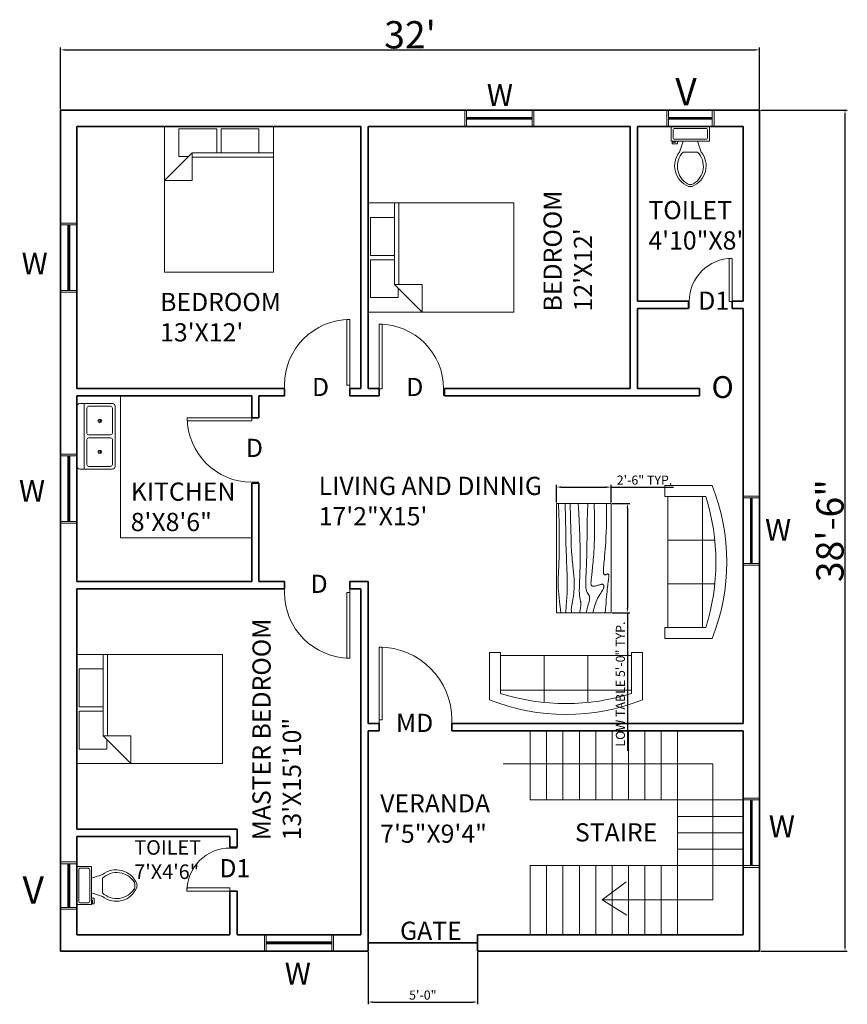
# Model space of a CAD drawing. Units: inches. Extents: x 1662 to 23131, y 1265 to 19127.
# Tile 4 of 26: x 8519 to 8974, y 5033 to 5574. Entities that reach past the tile are written whole.
import ezdxf

# ---------------------------------------------------------------- set-up
doc = ezdxf.new("R2010")
doc.units = ezdxf.units.IN
for name, color, linetype, lineweight in [('A-ANNO-DIMS', 4, 'Continuous', 18), ('A-ANNO-IDEN', 7, 'Continuous', 18), ('A-AREA-IDEN', 7, 'Continuous', 18), ('A-DOOR', 3, 'Continuous', 18), ('A-FLOR-CASE', 8, 'Continuous', 18), ('A-FLOR-FIXT', 9, 'Continuous', 18), ('A-FLOR-STRS', 7, 'Continuous', 18), ('A-FURN', 8, 'Continuous', 18), ('A-GLAZ', 4, 'Continuous', 18), ('A-WALL', 7, 'Continuous', 35)]:
    doc.layers.add(name, color=color, linetype=linetype, lineweight=lineweight)
doc.styles.get("Standard").update_dxf_attribs({"font": 'arial.ttf'})
doc.dimstyles.new('ISO-25', dxfattribs={"dimtxt": 5, "dimasz": 2.5, "dimexe": 1.25, "dimexo": 0.625, "dimtad": 1, "dimlunit": 3, "dimtxsty": 'Standard', "dimcen": 2.5, "dimadec": 0, "dimazin": 0, "dimtfac": 1, "dimtmove": 0, "dimatfit": 3, "dimfxl": 1, "dimarcsym": 0})

# ---------------------------------------------------------------- blocks, each defined once
blk = doc.blocks.new('Table - Rectangular Woodgrain 60 x 30 in.')
for p, q in [((0, 0), (0, -30)), ((60, 0), (0, 0)), ((60, -30), (60, 0)), ((0, -30), (60, -30))]:
    blk.add_line(p, q)
for points in [[(0, -2.4), (4.8155, -2.418), (9.0302, -2.4688), (12.709, -2.5477), (15.9167, -2.65), (18.7181, -2.7711), (21.1781, -2.9063), (23.3616, -3.0508), (25.3333, -3.2), (27.1477, -3.3495), (28.8172, -3.4958), (30.3437, -3.636), (31.7291, -3.7667), (32.9756, -3.8849), (34.0849, -3.9875), (35.059, -4.0714), (35.9, -4.1334), (36.6114, -4.1711), (37.2041, -4.1854), (37.6906, -4.1779), (38.0833, -4.15), (38.3948, -4.1034), (38.6375, -4.0396), (38.8239, -3.9602), (38.9666, -3.8667), (39.0764, -3.7608), (39.1573, -3.6448), (39.2116, -3.521), (39.2416, -3.3917), (39.2498, -3.2593), (39.2385, -3.1261), (39.21, -2.9944), (39.1666, -2.8667), (39.111, -2.7447), (39.0468, -2.6281), (38.978, -2.5163), (38.9083, -2.4083), (38.8418, -2.3035), (38.7823, -2.201), (38.7337, -2.1001), (38.7, -2), (38.6844, -1.9003), (38.6875, -1.8021), (38.7094, -1.707), (38.75, -1.6167), (38.8094, -1.5326), (38.8875, -1.4563), (38.9844, -1.3893), (39.1, -1.3333), (39.2351, -1.2896), (39.3937, -1.2583), (39.5804, -1.2396), (39.8, -1.2333), (40.057, -1.2396), (40.3562, -1.2583), (40.7023, -1.2896), (41.1, -1.3333), (41.5547, -1.3895), (42.0755, -1.4573), (42.6721, -1.5361), (43.3542, -1.625), (44.1316, -1.7233), (45.014, -1.8302), (46.0114, -1.9449), (47.1333, -2.0667), (48.3862, -2.1947), (49.7625, -2.3281), (51.2513, -2.4663), (52.8416, -2.6083), (54.5226, -2.7535), (56.2833, -2.9011), (58.1127, -3.0501), (60, -3.2)], [(0, -9.2), (6.5759, -9.0858), (11.9385, -9.0365), (16.2527, -9.0418), (19.6833, -9.0917), (22.3952, -9.1759), (24.5531, -9.2844), (26.322, -9.4069), (27.8666, -9.5333), (29.3241, -9.6553), (30.7203, -9.7719), (32.0532, -9.8837), (33.3208, -9.9917), (34.5213, -10.0965), (35.6526, -10.199), (36.7128, -10.2999), (37.7, -10.4), (38.6129, -10.4996), (39.4531, -10.5969), (40.223, -10.6895), (40.925, -10.775), (41.5613, -10.8512), (42.1344, -10.9156), (42.6465, -10.966), (43.1, -11), (43.4976, -11.0158), (43.8437, -11.0136), (44.143, -10.9942), (44.4, -10.9583), (44.6195, -10.9069), (44.8062, -10.8406), (44.9648, -10.7603), (45.1, -10.6667), (45.2155, -10.5598), (45.3114, -10.4365), (45.3871, -10.2929), (45.4416, -10.125), (45.4743, -9.929), (45.4844, -9.7011), (45.4709, -9.4371), (45.4333, -9.1333), (45.3716, -8.7883), (45.2896, -8.4104), (45.1919, -8.0107), (45.0833, -7.6), (44.9685, -7.1893), (44.8521, -6.7896), (44.7388, -6.4117), (44.6333, -6.0667), (44.54, -5.7628), (44.4614, -5.4979), (44.4001, -5.2675), (44.3583, -5.0667), (44.3384, -4.8909), (44.3427, -4.7354), (44.3736, -4.5956), (44.4333, -4.4667), (44.5236, -4.3453), (44.6427, -4.2333), (44.7884, -4.1339), (44.9583, -4.05), (45.1501, -3.9849), (45.3614, -3.9417), (45.59, -3.9234), (45.8333, -3.9333), (46.0915, -3.9749), (46.3734, -4.0531), (46.6906, -4.1736), (47.0542, -4.3417), (47.4756, -4.5629), (47.9661, -4.8427), (48.5372, -5.1866), (49.2, -5.6), (49.9676, -6.0844), (50.8594, -6.625), (51.8965, -7.2031), (53.1, -7.8), (54.491, -8.3969), (56.0906, -8.975), (57.9199, -9.5156), (60, -10)], [(0, -12.8), (5.1847, -12.9322), (9.6213, -13.0323), (13.3963, -13.1059), (16.5958, -13.1583), (19.3063, -13.1952), (21.614, -13.2219), (23.6054, -13.2439), (25.3666, -13.2667), (26.9728, -13.2947), (28.4531, -13.3281), (29.8256, -13.3663), (31.1083, -13.4083), (32.3191, -13.4535), (33.476, -13.501), (34.597, -13.5501), (35.7, -13.6), (36.7984, -13.6497), (37.8875, -13.6979), (38.9578, -13.743), (40, -13.7833), (41.0047, -13.8174), (41.9625, -13.8438), (42.864, -13.8607), (43.7, -13.8667), (44.4631, -13.8604), (45.1552, -13.8417), (45.7801, -13.8104), (46.3416, -13.7667), (46.8439, -13.7104), (47.2906, -13.6417), (47.6858, -13.5604), (48.0333, -13.4667), (48.3375, -13.3608), (48.6042, -13.2448), (48.8396, -13.121), (49.05, -12.9917), (49.2417, -12.8593), (49.4208, -12.7261), (49.5937, -12.5944), (49.7667, -12.4667), (49.9452, -12.3451), (50.1323, -12.2313), (50.3303, -12.1268), (50.5416, -12.0333), (50.7686, -11.9524), (51.0135, -11.8854), (51.2788, -11.8341), (51.5666, -11.8), (51.8785, -11.7843), (52.2116, -11.7865), (52.562, -11.8059), (52.926, -11.8417), (53.2998, -11.8931), (53.6795, -11.9594), (54.0614, -12.0397), (54.4416, -12.1333), (54.8223, -12.2401), (55.2293, -12.3625), (55.6942, -12.5037), (56.2489, -12.6667), (56.9251, -12.8547), (57.7545, -13.0708), (58.7689, -13.3182), (60, -13.6)], [(0, -18), (5.124, -17.7273), (9.6609, -17.5057), (13.6705, -17.3303), (17.2125, -17.1958), (20.3467, -17.0973), (23.1328, -17.0297), (25.6307, -16.9878), (27.9, -16.9667), (29.9928, -16.9617), (31.9302, -16.9703), (33.7254, -16.9907), (35.3917, -17.0208), (36.9423, -17.0588), (38.3906, -17.1026), (39.7499, -17.1503), (41.0333, -17.2), (42.2519, -17.2496), (43.4073, -17.2969), (44.4986, -17.3395), (45.525, -17.375), (46.4858, -17.4012), (47.3802, -17.4156), (48.2074, -17.416), (48.9667, -17.4), (49.6583, -17.3662), (50.2872, -17.3167), (50.8595, -17.2547), (51.3812, -17.1833), (51.8584, -17.1057), (52.2971, -17.025), (52.7034, -16.9443), (53.0833, -16.8667), (53.443, -16.7951), (53.789, -16.7313), (54.128, -16.6768), (54.4666, -16.6334), (54.8115, -16.6024), (55.1693, -16.5854), (55.5465, -16.5841), (55.95, -16.6), (56.3828, -16.6337), (56.8346, -16.6823), (57.2915, -16.7418), (57.7396, -16.8084), (58.165, -16.878), (58.5539, -16.9469), (58.8924, -17.0111), (59.1666, -17.0667), (59.3679, -17.1107), (59.5078, -17.1438), (59.6032, -17.1675), (59.6708, -17.1833), (59.7275, -17.193), (59.7901, -17.1979), (59.8753, -17.1998), (60, -17.2)], [(0, -22.4), (8.0098, -22.2501), (14.4094, -22.1011), (19.4168, -21.9535), (23.25, -21.8083), (26.1269, -21.6663), (28.2656, -21.5281), (29.884, -21.3947), (31.2, -21.2667), (32.3967, -21.1448), (33.5172, -21.0292), (34.5697, -20.9198), (35.5625, -20.8167), (36.5037, -20.7198), (37.4015, -20.6292), (38.2642, -20.5448), (39.1, -20.4667), (39.9164, -20.3951), (40.7187, -20.3313), (41.5117, -20.2768), (42.3, -20.2333), (43.0883, -20.2024), (43.8812, -20.1854), (44.6836, -20.1841), (45.5, -20.2), (46.3328, -20.234), (47.1747, -20.2844), (48.0163, -20.3488), (48.8479, -20.425), (49.66, -20.5106), (50.4429, -20.6031), (51.1872, -20.7004), (51.8833, -20.8), (52.5246, -20.8999), (53.1166, -20.9995), (53.6681, -21.0983), (54.1875, -21.1958), (54.6834, -21.2919), (55.1646, -21.3859), (55.6394, -21.4777), (56.1167, -21.5667), (56.6028, -21.6515), (57.0961, -21.7266), (57.5929, -21.7852), (58.0896, -21.8208), (58.5823, -21.8268), (59.0674, -21.7964), (59.5412, -21.723), (60, -21.6)], [(0, -25.2), (8.6355, -25.0504), (15.7026, -24.9031), (21.4049, -24.7606), (25.9458, -24.625), (29.529, -24.4988), (32.3578, -24.3844), (34.6359, -24.284), (36.5667, -24.2), (38.3213, -24.1341), (39.9417, -24.0854), (41.437, -24.0523), (42.8167, -24.0333), (44.0901, -24.0268), (45.2667, -24.0313), (46.3557, -24.0451), (47.3667, -24.0667), (48.309, -24.0947), (49.1928, -24.1287), (50.0284, -24.168), (50.826, -24.2125), (51.5959, -24.2617), (52.3483, -24.3151), (53.0935, -24.3725), (53.8417, -24.4334), (54.6009, -24.497), (55.3699, -24.561), (56.1454, -24.6226), (56.9239, -24.6792), (57.7021, -24.7279), (58.4764, -24.7662), (59.2435, -24.7911), (60, -24.8)], [(0, -28.8), (5.6867, -28.6681), (10.45, -28.5698), (14.407, -28.5012), (17.675, -28.4584), (20.3711, -28.4374), (22.6125, -28.4344), (24.5164, -28.4455), (26.2, -28.4667), (27.762, -28.4947), (29.2276, -28.5281), (30.6033, -28.5663), (31.8958, -28.6084), (33.1118, -28.6535), (34.2578, -28.7011), (35.3405, -28.7501), (36.3666, -28.8), (37.3443, -28.8497), (38.288, -28.8974), (39.2137, -28.9412), (40.1375, -28.9792), (41.0753, -29.0093), (42.0432, -29.0297), (43.0572, -29.0384), (44.1333, -29.0333), (45.2936, -29.0114), (46.5843, -28.9641), (48.0579, -28.8816), (49.7666, -28.7542), (51.7629, -28.5721), (54.0989, -28.3255), (56.8272, -28.0048), (60, -27.6)]]:
    blk.add_lwpolyline(points)
blk = doc.blocks.new('Bed - Queen')
for p, q in [((0, -80.00003), (0, 0)), ((0, 0), (59.99999, 0)), ((59.99999, 0), (59.99999, -80.00003)), ((7.99999, -1.2), (28.79998, -1.2)), ((7.99999, -14.4), (7.99999, -1.2)), ((28.79998, -1.2), (28.79998, -14.4)), ((31.19999, -1.2), (51.99999, -1.2)), ((31.19999, -14.4), (31.19999, -1.2)), ((51.99999, -1.2), (51.99999, -16.4)), ((0, -14.4), (44.8, -14.4)), ((59.99999, -29.6), (44.8, -14.4)), ((44.8, -14.4), (44.8, -29.6)), ((44.8, -16.8), (0, -16.8)), ((51.99999, -16.4), (46.79936, -16.4)), ((44.8, -29.6), (59.99999, -29.6)), ((59.99999, -80.00003), (0, -80.00003))]:
    blk.add_line(p, q)
blk = doc.blocks.new('*U33')
for p, q in [((0, 0), (0, -6)), ((40, 0), (40, -6))]:
    blk.add_line(p, q)
blk.add_lwpolyline([(0, 0), (0, 40), (1.75, 40), (1.75, 0)], close=True)
blk.add_arc((0, 0), 40, 0, 90)
blk = doc.blocks.new('*U34')
for p, q in [((0, 0), (0, -6)), ((-36, 0), (-36, -6))]:
    blk.add_line(p, q)
blk.add_lwpolyline([(0, 0), (0, 36), (-1.75, 36), (-1.75, 0)], close=True)
blk.add_arc((0, 0), 36, 90, 180)
blk = doc.blocks.new('*U40')
for p, q in [((-36, 0), (-36, 6)), ((0, 0), (0, 6))]:
    blk.add_line(p, q)
blk.add_lwpolyline([(0, 0), (0, -36), (-1.75, -36), (-1.75, 0)], close=True)
blk.add_arc((0, 0), 36, 180, 270)
blk = doc.blocks.new('*U42')
for p, q in [((0, 0), (0, -100)), ((900, 0), (900, -100))]:
    blk.add_line(p, q)
blk.add_lwpolyline([(0, 0), (0, 900), (43.75, 900), (43.75, 0)], close=True)
blk.add_arc((0, 0), 900, 0, 90)
blk = doc.blocks.new('*U41')
for p, q in [((0, 0), (0, -100)), ((-900, 0), (-900, -100))]:
    blk.add_line(p, q)
blk.add_lwpolyline([(0, 0), (0, 900), (-43.75, 900), (-43.75, 0)], close=True)
blk.add_arc((0, 0), 900, 90, 180)
blk = doc.blocks.new('*U35')
for p, q in [((0, 0), (0, -100)), ((600, 0), (600, -100))]:
    blk.add_line(p, q)
blk.add_lwpolyline([(0, 0), (0, 600), (43.75, 600), (43.75, 0)], close=True)
blk.add_arc((0, 0), 600, 0, 90)
blk = doc.blocks.new('*U43')
for p, q in [((-600, 0), (-600, -100)), ((0, 0), (0, -100))]:
    blk.add_line(p, q)
blk.add_lwpolyline([(0, 0), (0, 600), (-43.75, 600), (-43.75, 0)], close=True)
blk.add_arc((0, 0), 600, 90, 180)
blk = doc.blocks.new('Sofa - Roundback 7 ft.')
for p, q in [((-12.00002, -32.4421), (-12.00003, -6.5971)), ((11.99997, -32.4421), (11.99998, -6.5971)), ((-36.000027, -34), (-36.000027, -11.4696)), ((-35.999844, -13.3819), (35.9998, -13.3819)), ((35.99998, -34), (35.99998, -11.4696)), ((-36.000027, -32.4421), (35.99998, -32.4421))]:
    blk.add_line(p, q)
for points in [[(-36.000027, -34), (-42.000027, -34), (-42.000027, -8)], [(41.99998, -8), (41.99998, -34), (35.99998, -34)]]:
    blk.add_lwpolyline(points)
for centre, radius, start, end in [((0, -114.25), 114.25, 68.43141, 111.5686), ((-0.00001, -127.1968), 121.1968, 72.72033, 107.2797)]:
    blk.add_arc(centre, radius, start, end)
blk = doc.blocks.new('Toilet - top')
for p, q in [((9.5, -6), (9.5, -2)), ((-10, -8.5), (-8, -8.5)), ((-10, -9.5), (-10, -8.5)), ((-7, -9.5), (-10, -9.5)), ((-8, -8.5), (-8, -8)), ((-7, -8), (-7, -9.5)), ((-4, -8), (-6, -14)), ((4, -8), (6, -14)), ((4, -14), (-4, -14))]:
    blk.add_line(p, q)
blk.add_lwpolyline([(10.5, -8), (10.5, 0), (-10.5, 0), (-10.5, -8)], close=True)
for points in [[(-9.5, -2), (-9.5, -6)], [(8.5, -1), (-8.5, -1)], [(-8.5, -7), (8.5, -7)]]:
    blk.add_lwpolyline(points)
for centre, radius, start, end in [((-8.62, -1.88), 0.884, 81.8699, 188.1301), ((8.62, -1.88), 0.884, 351.8699, 98.1301), ((-8.62, -6.12), 0.884, 171.8699, 278.1301), ((8.62, -6.12), 0.884, 261.8699, 8.1301), ((3.52, -21.58), 12.17, 141.4691, 247.9714), ((4.2, -21.82), 11.33, 136.3677, 238.9468), ((-3.52, -21.58), 12.17, 292.0284, 38.5307), ((-4.2, -21.82), 11.33, 301.053, 43.6321), ((0, -27.88), 4, 245.7318, 294.2682), ((0, -29), 4, 254.8605, 285.1395)]:
    blk.add_arc(centre, radius, start, end)
blk = doc.blocks.new('Sink-double - 36 in top')
for p, q in [((-18, -4), (18, -4)), ((-0.75, -18.5), (-0.75, -6.5)), ((0.75, -6.5), (0.75, -18.5))]:
    blk.add_line(p, q)
for points in [[(-16.5, 0), (16.5, 0)], [(-18, -19.5), (-18, -1.5)], [(18, -1.5), (18, -19.5)], [(-16.5, -18.5), (-16.5, -6.5)], [(-15.5, -5.5), (-1.75, -5.5)], [(1.75, -5.5), (15.5, -5.5)], [(16.5, -6.5), (16.5, -18.5)], [(16.5, -21), (-16.5, -21)], [(-1.75, -19.5), (-15.5, -19.5)], [(15.5, -19.5), (1.75, -19.5)]]:
    blk.add_lwpolyline(points)
for centre, radius in [((-8.5, -12.5), 1), ((-8.5, -12.5), 0.5), ((8.5, -12.5), 1), ((8.5, -12.5), 0.5)]:
    blk.add_circle(centre, radius)
for centre, radius, start, end in [((-16.5, -1.5), 1.5, 90, 180), ((16.5, -1.5), 1.5, 0, 90), ((-15.5, -6.5), 1, 90, 180), ((-1.75, -6.5), 1, 0, 90), ((1.75, -6.5), 1, 90, 180), ((15.5, -6.5), 1, 0, 90), ((-16.5, -19.5), 1.5, 180, 270), ((-15.5, -18.5), 1, 180, 270), ((-1.75, -18.5), 1, 270, 0), ((1.75, -18.5), 1, 180, 270), ((15.5, -18.5), 1, 270, 0), ((16.5, -19.5), 1.5, 270, 0)]:
    blk.add_arc(centre, radius, start, end)
blk = doc.blocks.new('*D44')
at = {"layer": 'A-ANNO-DIMS', "color": 0, "lineweight": -2, "transparency": 16777216}
for p, q in [((8541.92, 5525.22), (8541.92, 5558.98)), ((8544.42, 5557.73), (8923.42, 5557.73)), ((8925.92, 5525.22), (8925.92, 5558.98))]:
    blk.add_line(p, q, dxfattribs=at)
at = {"layer": 'A-ANNO-DIMS', "color": 0, "transparency": 16777216}
for points in [[(8544.42, 5558.15), (8544.42, 5557.32), (8541.92, 5557.73)], [(8923.42, 5558.15), (8923.42, 5557.32), (8925.92, 5557.73)]]:
    blk.add_solid(points, dxfattribs=at)
at = {"layer": 'Defpoints', "color": 0, "transparency": 16777216}
for p in [(8925.92, 5557.73), (8541.92, 5524.6), (8925.92, 5524.6)]:
    blk.add_point(p, dxfattribs=at)
at = {"layer": 'A-ANNO-DIMS', "color": 0, "transparency": 16777216, "insert": (8733.92, 5566.02), "char_height": 5, "attachment_point": 5}
blk.add_mtext("{\\H3x;32'}", dxfattribs=at)
blk = doc.blocks.new('*D45')
at = {"layer": 'A-ANNO-DIMS', "color": 0, "lineweight": -2, "transparency": 16777216}
for p, q in [((8926.55, 5524.6), (8974.14, 5524.6)), ((8972.89, 5065.1), (8972.89, 5522.1)), ((8926.55, 5062.6), (8974.14, 5062.6))]:
    blk.add_line(p, q, dxfattribs=at)
at = {"layer": 'A-ANNO-DIMS', "color": 0, "transparency": 16777216}
for points in [[(8972.48, 5522.1), (8973.31, 5522.1), (8972.89, 5524.6)], [(8972.48, 5065.1), (8973.31, 5065.1), (8972.89, 5062.6)]]:
    blk.add_solid(points, dxfattribs=at)
at = {"layer": 'Defpoints', "color": 0, "transparency": 16777216}
for p in [(8925.92, 5524.6), (8972.89, 5524.6), (8925.92, 5062.6)]:
    blk.add_point(p, dxfattribs=at)
at = {"layer": 'A-ANNO-DIMS', "color": 0, "transparency": 16777216, "insert": (8964.61, 5293.6), "char_height": 5, "attachment_point": 5, "rotation": 90}
blk.add_mtext('{\\H3x;38\'-6"}', dxfattribs=at)
blk = doc.blocks.new('WIN-36-J9X1')
for p, q in [((0, 9), (0, 0)), ((1, 9), (1, 0)), ((37, 9), (37, 0)), ((38, 9), (38, 0)), ((1, 5), (37, 5)), ((1, 4.5), (37, 4.5)), ((1, 4), (37, 4))]:
    blk.add_line(p, q)
blk = doc.blocks.new('VENT-24-J9X1')
for p, q in [((0, 9), (0, 0)), ((1, 9), (1, 0)), ((25, 9), (25, 0)), ((26, 9), (26, 0)), ((1, 5), (25, 5)), ((1, 4.5), (25, 4.5)), ((1, 4), (25, 4))]:
    blk.add_line(p, q)
blk = doc.blocks.new('*D169')
at = {"layer": 'A-ANNO-DIMS', "color": 0, "lineweight": -2, "transparency": 16777216}
for p, q in [((8844.96, 5308.51), (8854.58, 5308.51)), ((8853.33, 5306.01), (8853.33, 5251.01)), ((8844.96, 5248.51), (8854.58, 5248.51)), ((8853.33, 5248.51), (8853.33, 5172.58))]:
    blk.add_line(p, q, dxfattribs=at)
at = {"layer": 'A-ANNO-DIMS', "color": 0, "transparency": 16777216}
for points in [[(8852.91, 5306.01), (8853.75, 5306.01), (8853.33, 5308.51)], [(8852.91, 5251.01), (8853.75, 5251.01), (8853.33, 5248.51)]]:
    blk.add_solid(points, dxfattribs=at)
at = {"layer": 'Defpoints', "color": 0, "transparency": 16777216}
for p in [(8844.33, 5308.51), (8844.33, 5248.51), (8853.33, 5248.51)]:
    blk.add_point(p, dxfattribs=at)
at = {"layer": 'A-ANNO-DIMS', "color": 0, "transparency": 16777216, "insert": (8850.12, 5209.29), "char_height": 5, "attachment_point": 5, "rotation": 90}
blk.add_mtext('LOW TABLE 5\'-0" TYP.', dxfattribs=at)
blk = doc.blocks.new('*D170')
at = {"layer": 'A-ANNO-DIMS', "color": 0, "lineweight": -2, "transparency": 16777216}
for p, q in [((8814.33, 5309.13), (8814.33, 5318.76)), ((8844.33, 5309.13), (8844.33, 5318.76)), ((8816.83, 5317.51), (8841.83, 5317.51)), ((8844.33, 5317.51), (8878.64, 5317.51))]:
    blk.add_line(p, q, dxfattribs=at)
at = {"layer": 'A-ANNO-DIMS', "color": 0, "transparency": 16777216}
for points in [[(8816.83, 5317.92), (8816.83, 5317.09), (8814.33, 5317.51)], [(8841.83, 5317.92), (8841.83, 5317.09), (8844.33, 5317.51)]]:
    blk.add_solid(points, dxfattribs=at)
at = {"layer": 'Defpoints', "color": 0, "transparency": 16777216}
for p in [(8844.33, 5317.51), (8814.33, 5308.51), (8844.33, 5308.51)]:
    blk.add_point(p, dxfattribs=at)
at = {"layer": 'A-ANNO-DIMS', "color": 0, "transparency": 16777216, "insert": (8862.74, 5320.69), "char_height": 5, "attachment_point": 5}
blk.add_mtext('2\'-6" TYP.', dxfattribs=at)
blk = doc.blocks.new('*D208')
at = {"layer": 'A-ANNO-DIMS', "color": 0, "lineweight": -2, "transparency": 16777216}
for p, q in [((8710.92, 5061.97), (8710.92, 5033.35)), ((8770.92, 5061.97), (8770.92, 5033.35)), ((8713.42, 5034.6), (8768.42, 5034.6))]:
    blk.add_line(p, q, dxfattribs=at)
at = {"layer": 'A-ANNO-DIMS', "color": 0, "transparency": 16777216}
for points in [[(8713.42, 5035.01), (8713.42, 5034.18), (8710.92, 5034.6)], [(8768.42, 5035.01), (8768.42, 5034.18), (8770.92, 5034.6)]]:
    blk.add_solid(points, dxfattribs=at)
at = {"layer": 'Defpoints', "color": 0, "transparency": 16777216}
for p in [(8710.92, 5062.6), (8770.92, 5062.6), (8770.92, 5034.6)]:
    blk.add_point(p, dxfattribs=at)
at = {"layer": 'A-ANNO-DIMS', "color": 0, "transparency": 16777216, "insert": (8740.92, 5037.77), "char_height": 5, "attachment_point": 5}
blk.add_mtext('5\'-0"', dxfattribs=at)

msp = doc.modelspace()

# ---------------------------------------------------------------- linework, layer by layer
at = {"layer": 'A-FLOR-CASE'}
for q in [(8574.923, 5367.596), (8646.923, 5289.596)]:
    msp.add_line((8574.923, 5289.596), q, dxfattribs=at)
at = {"layer": 'A-FLOR-STRS'}
for p, q in [((8799.923, 5183.596), (8799.923, 5145.596)), ((8808.923, 5183.596), (8808.923, 5145.596)), ((8817.923, 5183.596), (8817.923, 5145.596)), ((8826.923, 5183.596), (8826.923, 5145.596)), ((8835.923, 5183.596), (8835.923, 5145.596)), ((8844.923, 5183.596), (8844.923, 5145.596)), ((8853.923, 5183.596), (8853.923, 5145.596)), ((8862.923, 5183.596), (8862.923, 5145.596)), ((8871.923, 5183.596), (8871.923, 5145.596)), ((8880.923, 5183.596), (8880.923, 5071.596)), ((8785.065, 5165.446), (8900.216, 5165.446)), ((8900.216, 5165.446), (8900.216, 5090.803)), ((8916.923, 5145.596), (8799.923, 5145.596)), ((8916.923, 5136.596), (8880.923, 5136.596)), ((8916.923, 5127.596), (8880.923, 5127.596)), ((8916.923, 5118.596), (8880.923, 5118.596)), ((8916.923, 5109.596), (8799.923, 5109.596)), ((8799.923, 5109.596), (8799.923, 5071.596)), ((8808.923, 5109.596), (8808.923, 5071.596)), ((8817.923, 5109.596), (8817.923, 5071.596)), ((8826.923, 5109.596), (8826.923, 5071.596)), ((8835.923, 5109.596), (8835.923, 5071.596)), ((8844.923, 5109.596), (8844.923, 5071.596)), ((8853.923, 5109.596), (8853.923, 5071.596)), ((8862.923, 5109.596), (8862.923, 5071.596)), ((8871.923, 5109.596), (8871.923, 5071.596)), ((8839.447, 5090.803), (8852.674, 5100.631)), ((8900.216, 5090.803), (8839.447, 5090.803)), ((8839.447, 5090.803), (8853.037, 5082.411))]:
    msp.add_line(p, q, dxfattribs=at)
at = {"layer": 'A-WALL'}
for p, q in [((8541.923, 5524.596), (8925.923, 5524.596)), ((8541.923, 5062.596), (8541.923, 5524.596)), ((8925.923, 5524.596), (8925.923, 5062.596)), ((8550.923, 5515.596), (8706.923, 5515.596)), ((8550.923, 5371.596), (8550.923, 5515.596)), ((8706.923, 5371.596), (8706.923, 5515.596)), ((8710.923, 5371.596), (8710.923, 5515.596)), ((8710.923, 5515.596), (8854.923, 5515.596)), ((8854.923, 5371.596), (8854.923, 5515.596)), ((8858.923, 5419.596), (8858.923, 5515.596)), ((8858.923, 5515.596), (8916.923, 5515.596)), ((8916.923, 5515.596), (8916.923, 5419.596)), ((8858.923, 5419.596), (8886.923, 5419.596)), ((8858.923, 5371.596), (8858.923, 5415.596)), ((8858.923, 5415.596), (8886.923, 5415.596)), ((8886.923, 5419.596), (8886.923, 5415.596)), ((8910.923, 5419.596), (8910.923, 5415.596)), ((8910.923, 5419.596), (8916.923, 5419.596)), ((8910.923, 5415.596), (8916.923, 5415.596)), ((8916.923, 5415.596), (8916.923, 5187.596)), ((8550.923, 5371.596), (8664.923, 5371.596)), ((8550.923, 5367.596), (8646.923, 5367.596)), ((8550.923, 5265.596), (8550.923, 5367.596)), ((8550.923, 5367.596), (8550.923, 5335.596)), ((8646.923, 5355.596), (8646.923, 5367.596)), ((8650.923, 5355.596), (8650.923, 5367.596)), ((8650.923, 5367.596), (8664.923, 5367.596)), ((8664.923, 5371.596), (8664.923, 5367.596)), ((8700.923, 5371.596), (8700.923, 5367.596)), ((8700.923, 5371.596), (8706.923, 5371.596)), ((8700.923, 5367.596), (8716.923, 5367.596)), ((8710.923, 5371.596), (8716.923, 5371.596)), ((8716.923, 5371.596), (8716.923, 5367.596)), ((8752.923, 5371.596), (8752.923, 5367.596)), ((8752.923, 5371.596), (8854.923, 5371.596)), ((8752.923, 5367.596), (8892.923, 5367.596)), ((8858.923, 5371.596), (8892.923, 5371.596)), ((8892.923, 5371.596), (8892.923, 5367.596)), ((8646.923, 5355.596), (8650.923, 5355.596)), ((8646.923, 5265.596), (8646.923, 5319.596)), ((8646.923, 5319.596), (8650.923, 5319.596)), ((8650.923, 5265.596), (8650.923, 5319.596)), ((8550.923, 5265.596), (8646.923, 5265.596)), ((8650.923, 5265.596), (8664.923, 5265.596)), ((8664.923, 5261.596), (8664.923, 5265.596)), ((8700.923, 5261.596), (8700.923, 5265.596)), ((8700.923, 5265.596), (8710.923, 5265.596)), ((8710.923, 5187.596), (8710.923, 5265.596)), ((8550.923, 5261.596), (8664.923, 5261.596)), ((8550.923, 5129.596), (8550.923, 5261.596)), ((8700.923, 5261.596), (8706.923, 5261.596)), ((8706.923, 5071.596), (8706.923, 5261.596)), ((8716.923, 5187.596), (8710.923, 5187.596)), ((8710.923, 5062.596), (8710.923, 5183.596)), ((8716.923, 5183.596), (8710.923, 5183.596)), ((8716.923, 5183.596), (8716.923, 5187.596)), ((8916.923, 5187.596), (8756.923, 5187.596)), ((8756.923, 5183.596), (8756.923, 5187.596)), ((8916.923, 5183.596), (8756.923, 5183.596)), ((8916.923, 5183.596), (8916.923, 5071.596)), ((8638.923, 5129.596), (8550.923, 5129.596)), ((8638.923, 5119.596), (8638.923, 5129.596)), ((8550.923, 5071.596), (8550.923, 5125.596)), ((8634.923, 5125.596), (8550.923, 5125.596)), ((8634.923, 5119.596), (8634.923, 5125.596)), ((8638.923, 5119.596), (8634.923, 5119.596)), ((8634.923, 5071.596), (8634.923, 5095.596)), ((8638.923, 5095.596), (8634.923, 5095.596)), ((8638.923, 5071.596), (8638.923, 5095.596)), ((8634.923, 5071.596), (8550.923, 5071.596)), ((8706.923, 5071.596), (8638.923, 5071.596)), ((8916.923, 5071.596), (8770.923, 5071.596)), ((8770.923, 5062.596), (8770.923, 5071.596)), ((8770.923, 5067.096), (8710.923, 5067.096)), ((8710.923, 5062.596), (8541.923, 5062.596)), ((8925.923, 5062.596), (8770.923, 5062.596))]:
    msp.add_line(p, q, dxfattribs=at)

# ---------------------------------------------------------------- block references
at = {"layer": 'A-DOOR', "xscale": 0.0393700787401575, "yscale": 0.0393700787401575, "zscale": 0.0393700787401575}
for name, p in [('*U43', (8910.923, 5419.533)), ('*U42', (8716.923, 5371.533))]:
    msp.add_blockref(name, p, dxfattribs=at)
at = {"layer": 'A-DOOR'}
for name, p in [('*U34', (8700.923, 5373.596)), ('*U40', (8700.923, 5259.596)), ('*U33', (8716.923, 5189.596))]:
    msp.add_blockref(name, p, dxfattribs=at)
at = {"layer": 'A-DOOR', "xscale": 0.0393700787401575, "yscale": 0.0393700787401575, "zscale": 0.0393700787401575, "rotation": 89.99999999999996}
for name, p in [('*U41', (8646.986, 5355.596)), ('*U35', (8634.986, 5095.596))]:
    msp.add_blockref(name, p, dxfattribs=at)
at = {"layer": 'A-FLOR-FIXT'}
msp.add_blockref('Toilet - top', (8887.923, 5515.596), dxfattribs=at)
for name, p, rotation in [('Sink-double - 36 in top', (8550.923, 5345.384), 90), ('Toilet - top', (8550.923, 5098.596), 89.99999999999999)]:
    msp.add_blockref(name, p, dxfattribs=dict(at, rotation=rotation))
at = {"layer": 'A-FURN', "xscale": -1}
msp.add_blockref('Bed - Queen', (8658.923, 5515.596), dxfattribs=at)
at = {"layer": 'A-FURN', "xscale": -1, "rotation": 90}
for p in [(8710.923, 5473.596), (8550.923, 5225.596)]:
    msp.add_blockref('Bed - Queen', p, dxfattribs=at)
at = {"layer": 'A-FURN'}
for name, p, rotation in [('Sofa - Roundback 7 ft.', (8907.926, 5276.305), 269.9999999999999), ('Table - Rectangular Woodgrain 60 x 30 in.', (8844.331, 5308.508), 270), ('Sofa - Roundback 7 ft.', (8819.626, 5192.612), 179.9999999999999)]:
    msp.add_blockref(name, p, dxfattribs=dict(at, rotation=rotation))
at = {"layer": 'A-GLAZ'}
for name, p in [('WIN-36-J9X1', (8763.924, 5515.596)), ('VENT-24-J9X1', (8874.924, 5515.596)), ('WIN-36-J9X1', (8653.924, 5062.596))]:
    msp.add_blockref(name, p, dxfattribs=at)
at = {"layer": 'A-GLAZ', "rotation": 90}
for name, p in [('WIN-36-J9X1', (8550.924, 5424.596)), ('WIN-36-J9X1', (8550.924, 5297.596)), ('WIN-36-J9X1', (8925.924, 5274.596)), ('WIN-36-J9X1', (8925.924, 5108.596)), ('VENT-24-J9X1', (8550.924, 5085.596))]:
    msp.add_blockref(name, p, dxfattribs=at)

# ---------------------------------------------------------------- texts
at = {"layer": 'A-ANNO-IDEN', "attachment_point": 1}
for s, width, heights, insert, char_height in [('V', 1142.59551, [20], (8879.643, 5542.22), 15), ('W', 471.52273, [28.462], (8776.076, 5538.899), 12), ('W', 471.52273, [28.462], (8520.504, 5446.35), 12), ('D1', 1142.59551, [20], (8892.26, 5424.915), 10), ('D', 1142.59551, [0], (8680.048, 5377.496), 10), ('D', 1142.59551, [0], (8731.841, 5377.496), 10), ('O', 471.52273, [28.462], (8899.593, 5378.454), 12), ('D', 1142.59551, [0], (8643.753, 5344.041), 10), ('W', 471.52273, [28.462], (8519.031, 5321.463), 12), ('W', 471.52273, [28.462], (8928.935, 5300.05), 12), ('D', 1142.59551, [0], (8679.277, 5269.351), 10), ('MD', 1142.59551, [0], (8726.183, 5192.945), 10), ('W', 471.52273, [28.462], (8931.008, 5137.107), 12), ('D1', 1142.59551, [20], (8629.172, 5113.12), 10), ('V', 1142.59551, [20], (8521.006, 5103.625), 15), ('W', 471.52273, [28.462], (8665.066, 5056.228), 12)]:
    msp.add_mtext_dynamic_manual_height_columns(s, width=width, gutter_width=12.5, heights=heights, dxfattribs=dict(at, insert=insert, char_height=char_height))
at = {"layer": 'A-AREA-IDEN', "char_height": 10, "attachment_point": 1, "rotation": 90}
for s, insert in [("BEDROOM\\P12'X12'", (8807.258, 5414.03)), ('MASTER BEDROOM\\P13\'X15\'10"', (8647.327, 5123.433))]:
    msp.add_mtext_dynamic_manual_height_columns(s, width=1142.59551, gutter_width=12.5, heights=[277.772], dxfattribs=dict(at, insert=insert))
at = {"layer": 'A-AREA-IDEN', "attachment_point": 1}
for s, heights, insert, char_height in [('TOILET \\P4\'10"X8\'', [277.772], (8864.867, 5474.686), 10), ("BEDROOM\\P13'X12'", [277.772], (8596.599, 5424.199), 10), ('LIVING AND DINNIG\\P17\'2"X15\'', [277.772], (8683.731, 5323.167), 10), ('KITCHEN\\P8\'X8\'6"', [277.772], (8580.456, 5320.009), 10), ('VERANDA\\P7\'5"X9\'4"', [277.772], (8717.512, 5148.757), 10), ('STAIRE ', [0], (8824.508, 5132.803), 10), ('TOILET \\P7\'X4\'6"', [277.772], (8582.378, 5123.522), 8), ('GATE', [0], (8728.4, 5078.757), 10)]:
    msp.add_mtext_dynamic_manual_height_columns(s, width=1142.59551, gutter_width=12.5, heights=heights, dxfattribs=dict(at, insert=insert, char_height=char_height))

# ---------------------------------------------------------------- dimensions: what is measured, and where the dimension line sits
at = {"layer": 'A-ANNO-DIMS'}
dim = msp.add_linear_dim(base=(8925.923, 5557.732), p1=(8541.923, 5524.596), p2=(8925.923, 5524.596), text='{\\H3x;<>}', dimstyle='ISO-25', override={"dimclrd": 0, "dimclre": 0, "dimclrt": 0}, dxfattribs=at)
dim.commit()
dim.dimension.update_dxf_attribs({"geometry": '*D44', "text_midpoint": (8733.923, 5557.732), "dimtype": 160})
for base, p1, p2, angle, text, override, picture, middle in [((8972.895, 5524.596), (8925.923, 5062.596), (8925.923, 5524.596), 90, '{\\H3x;<>}', {"dimclrd": 0, "dimclre": 0, "dimclrt": 0}, '*D45', (8964.606, 5293.596)), ((8853.331, 5248.508), (8844.331, 5308.508), (8844.331, 5248.508), 270, 'LOW TABLE <> TYP.', {"dimdec": 1, "dimlfac": 1, "dimrnd": 0, "dimzin": 1, "dimdsep": 46, "dimlunit": 4, "dimfrac": 2}, '*D169', (8850.119, 5209.295))]:
    dim = msp.add_linear_dim(base=base, p1=p1, p2=p2, angle=angle, text=text, dimstyle='ISO-25', override=override, dxfattribs=at)
    dim.commit()
    dim.dimension.update_dxf_attribs({"geometry": picture, "text_midpoint": middle})
dim = msp.add_linear_dim(base=(8844.331, 5317.508), p1=(8814.331, 5308.508), p2=(8844.331, 5308.508), text='<> TYP.', dimstyle='ISO-25', override={"dimdec": 1, "dimlfac": 1, "dimrnd": 0, "dimzin": 1, "dimdsep": 46, "dimlunit": 4, "dimfrac": 2}, dxfattribs=at)
dim.commit()
dim.dimension.update_dxf_attribs({"geometry": '*D170', "text_midpoint": (8862.738, 5320.686)})
dim = msp.add_linear_dim(base=(8770.923, 5034.596), p1=(8710.923, 5062.596), p2=(8770.923, 5062.596), dimstyle='ISO-25', override={"dimdec": 1, "dimlfac": 1, "dimrnd": 0, "dimzin": 1, "dimdsep": 46, "dimlunit": 4, "dimfrac": 2}, dxfattribs=at)
dim.commit()
dim.dimension.update_dxf_attribs({"geometry": '*D208', "text_midpoint": (8740.923, 5037.774)})

doc.saveas('drawing.dxf')
